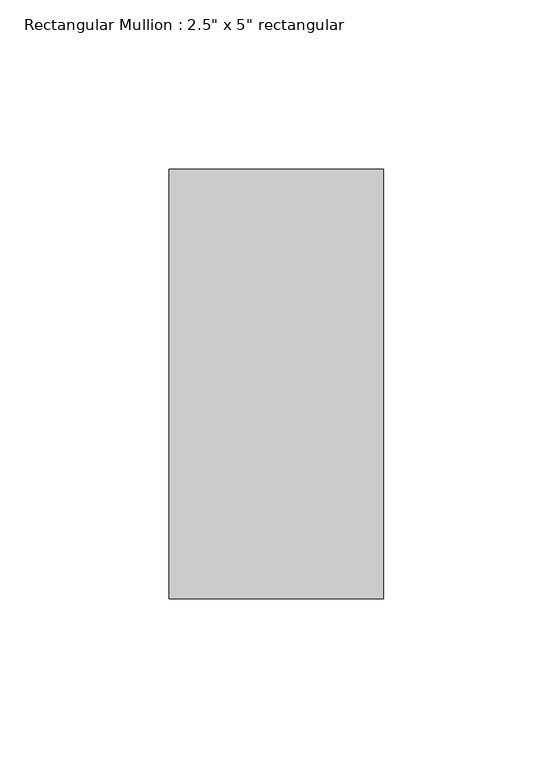
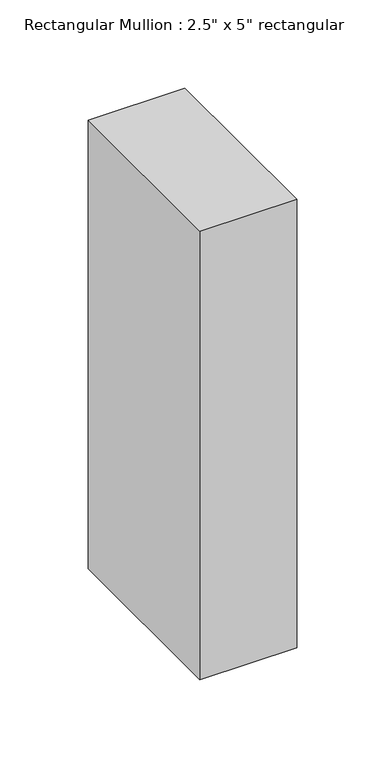
"""IFC4 building model written with IfcOpenShell, lengths in millimetres: member geometry."""

from ifc_helpers import new_model, si_unit, frame, origin, place, context, project, spatial, polyline, outline, extrude, source, transform, mapped, element, save


def member_5ad95953(model_context):
    return source(origin(), model_context, "Body", "SweptSolid", [
        extrude(outline(polyline([(0.0, 63.5), (0.0, -63.5), (-63.5, -63.5), (-63.5, 63.5), (0.0, 63.5)])), frame((0.0, 0.0, -311.15), z_axis=(0.0, 0.0, 1.0), x_axis=(1.0, 0.0, 0.0)), (0.0, 0.0, 1.0), 311.15),
    ])


if __name__ == "__main__":
    model = new_model("IFC4")
    model_context = context("Model", 3, world=origin())
    ifc_project = project(units=[si_unit("LENGTHUNIT", "METRE", prefix="MILLI")], contexts=[model_context])
    site = spatial("IfcSite", under=ifc_project)
    building = spatial("IfcBuilding", under=site)
    placement = place(None, origin())
    member_shape = member_5ad95953(model_context)
    element("IfcMember", 1, ObjectType="Rectangular Mullion : 2.5\" x 5\" rectangular", at=placement, inside=building, context=model_context, shape_type="MappedRepresentation", body=[
        mapped(member_shape, transform((0.0, 0.0, 0.0), x_axis=(1.0, 0.0, 0.0), y_axis=(0.0, 1.0, 0.0), z_axis=(0.0, 0.0, 1.0))),
    ])
    save(model, "model.ifc")

# Revit data of these elements
# Type "Rectangular Mullion : 2.5\" x 5\" rectangular"
#   built-in parameter 1007304 = 0.416667 (stored number, unit not read)
#   built-in parameter 1007301 = 0.104167 (stored number, unit not read)
#   built-in parameter 1007300 = 0.104167 (stored number, unit not read)
